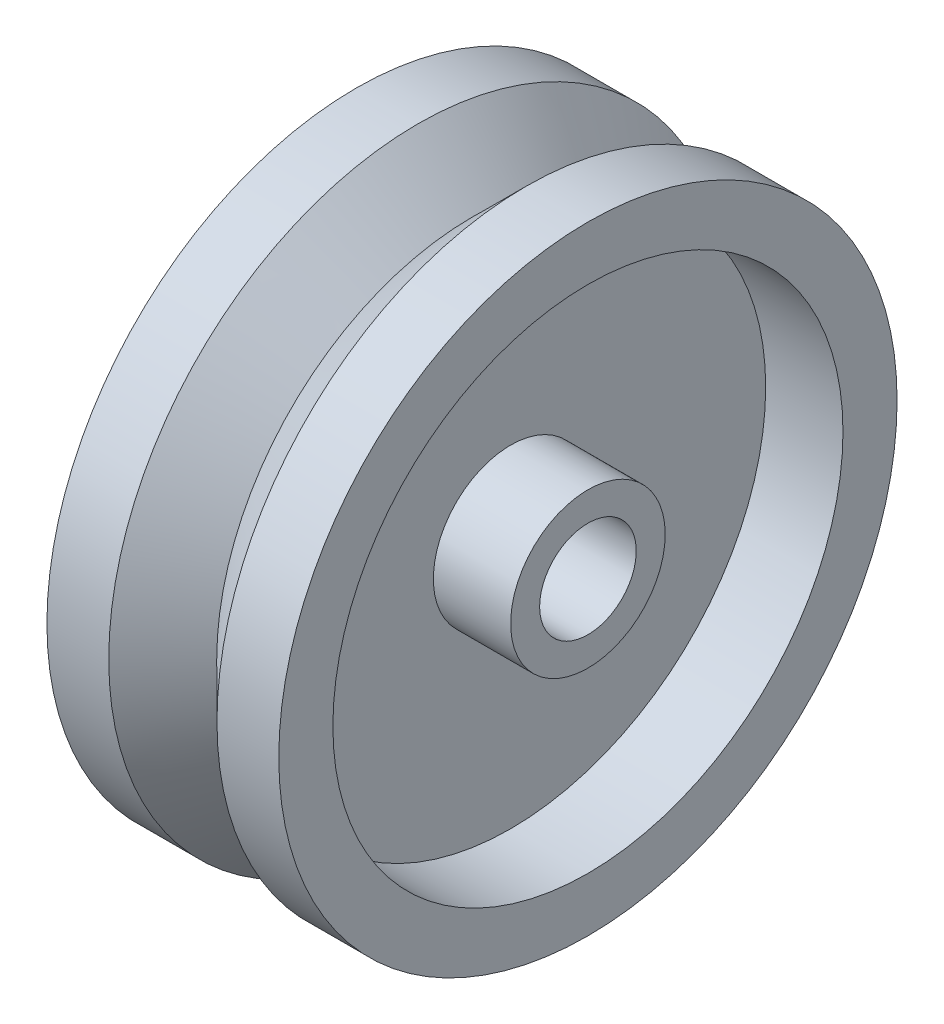
from build123d import *

# Parameters (mm, degrees)
SIDE_RECESS_SKETCH_33_R   = 16.5
SIDE_RECESS_SKETCH_33_R_2 = 5
SIDE_RECESS_33X5_DEPTH    = 5


with BuildPart() as part:
    # Wheel Profile Sketch → Wheel Body (revolve)
    with BuildSketch(Plane.XY, mode=Mode.PRIVATE) as wheel_body_sk:
        Polygon((-7.5, -3.125), (7.5, -3.125), (7.5, -20), (3.5, -20), (0, -16.514784956), (-3.5, -20), (-7.5, -20), align=None)
    revolve(wheel_body_sk.sketch.rotate(Axis((0, 0, 0), (1, 0, 0)), 270), axis=Axis((0, 0, 0), (1, 0, 0)))

    # Side Recess Sketch Ø33 → Side Recess Ø33x5 (cut)
    with BuildSketch(Plane(origin=(7.5, 0, 0), x_dir=(0, 0, -1), z_dir=(1, 0, 0))):
        Circle(SIDE_RECESS_SKETCH_33_R)
        Circle(SIDE_RECESS_SKETCH_33_R_2, mode=Mode.SUBTRACT)
    side_recess_33x5 = extrude(amount=-SIDE_RECESS_33X5_DEPTH, mode=Mode.SUBTRACT)

    # Side Recess Mirror: Side Recess Ø33x5 across plane
    add(side_recess_33x5.mirror(Plane(origin=(0, 0, 0), x_dir=(0, 0, 1), z_dir=(1, 0, 0))), mode=Mode.SUBTRACT)


solid = part.part
